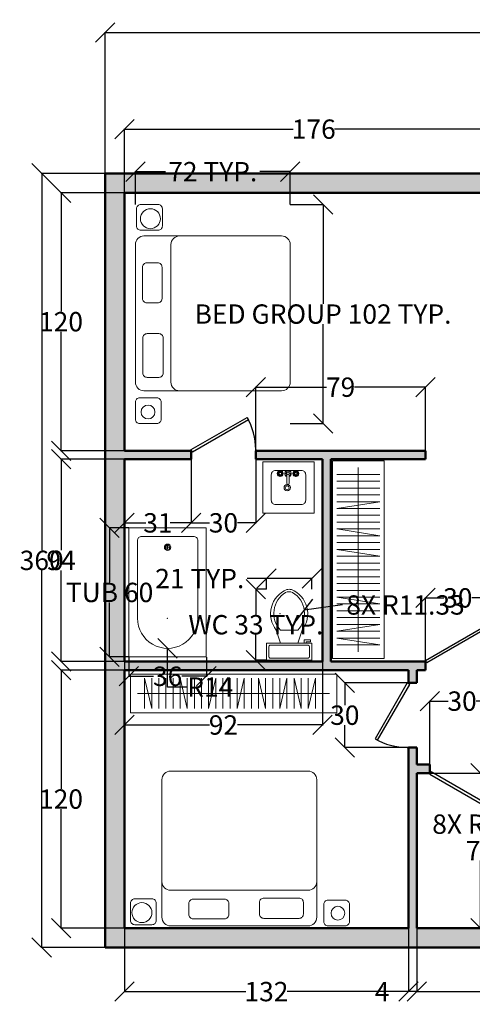
# Model space of a CAD drawing. Units: inches. Extents: x -9 to 615, y -420 to 89.
# Tile 1 of 6: x -9 to 201, y -368 to 89. Entities that reach past the tile are written whole.
import ezdxf

# ---------------------------------------------------------------- set-up
doc = ezdxf.new("R2010")
doc.units = ezdxf.units.IN
doc.header["$MEASUREMENT"] = 0
for name, color, linetype, lineweight in [('A-ANNO-DIMS', 2, 'Continuous', 18), ('A-DOOR', 4, 'Continuous', 25), ('A-FLOR-CASE', 32, 'Continuous', 18), ('A-FLOR-FIXT', 9, 'Continuous', 18), ('A-FURN', 8, 'Continuous', 18), ('A-WALL', 7, 'Continuous', 50)]:
    doc.layers.add(name, color=color, linetype=linetype, lineweight=lineweight)
doc.layers.add('A-WALL-PATT', color=251, linetype='Continuous', lineweight=13, true_color=0x636466)
doc.styles.get("Standard").update_dxf_attribs({"font": 'arial.ttf'})
doc.dimstyles.get("Standard").update_dxf_attribs({"dimtxt": 9, "dimasz": 9, "dimexe": 0.18, "dimexo": 0.0625, "dimgap": 0.09, "dimtad": 0, "dimtih": 1, "dimtoh": 1, "dimdec": 0, "dimzin": 0, "dimdsep": 46, "dimlunit": 4, "dimtxsty": 'Standard', "dimblk": 'OBLIQUE', "dimblk2": 'OBLIQUE', "dimcen": 0.09, "dimadec": 0, "dimazin": 0, "dimtfac": 1, "dimtdec": 0, "dimtofl": 0, "dimtmove": 0, "dimatfit": 3, "dimldrblk": 'OBLIQUE', "dimfxl": 1, "dimtolj": 1, "dimtzin": 0, "dimarcsym": 0})

# ---------------------------------------------------------------- blocks, each defined once
blk = doc.blocks.new('6 BED')
for p, q in [((-33.45, 25.64), (30.55, 25.64)), ((-37.45, 21.64), (-37.45, -23.43)), ((34.55, 21.64), (34.55, -19.64))]:
    blk.add_line(p, q)
for points in [[(-42.69, 42.2), (-50.69, 42.2, 0.414214), (-52.69, 40.2), (-52.69, 32.2, 0.414214), (-50.69, 30.2), (-42.69, 30.2, 0.414214), (-40.69, 32.2), (-40.69, 40.2, 0.414214)], [(-33.45, 42.2), (30.55, 42.2, -0.414214), (34.55, 38.2), (34.55, -25.8, -0.414214), (30.55, -29.8), (-33.45, -29.8, -0.414214), (-37.45, -25.8), (-37.45, 38.2, -0.414214)], [(39.19, 41.65), (47.19, 41.65, -0.414214), (49.19, 39.65), (49.19, 31.65, -0.414214), (47.19, 29.65), (39.19, 29.65, -0.414214), (37.19, 31.65), (37.19, 39.65, -0.414214)], [(-29.22, 38.71), (-12.85, 38.71, -0.414214), (-10.85, 36.71), (-10.85, 31.26, -0.414214), (-12.85, 29.26), (-29.22, 29.26, -0.414214), (-31.22, 31.26), (-31.22, 36.71, -0.414214)], [(5.45, 38.89), (20.03, 38.89, -0.414214), (22.03, 36.89), (22.03, 31.79, -0.414214), (20.03, 29.79), (5.45, 29.79, -0.414214), (3.45, 31.79), (3.45, 36.89, -0.414214)]]:
    blk.add_lwpolyline(points, format="xyb", close=True)
for centre, start, end in [((-33.45, 21.64), 90, 180), ((30.55, 21.64), 0, 90)]:
    blk.add_arc(centre, 4, start, end)
blk = doc.blocks.new('Bath Tub - 26 x 60 in.')
for p, q in [((8, -18), (10, -18)), ((9, -17), (9, -19))]:
    blk.add_line(p, q)
blk.add_lwpolyline([(0, -36), (0, 0), (60, 0), (60, -36)], close=True)
for points in [[(6, -4), (42, -4)], [(4, -30), (4, -6)], [(42, -32), (6, -32)]]:
    blk.add_lwpolyline(points)
for radius in [1.5, 1]:
    blk.add_circle((9, -18), radius)
for centre, radius, start, end in [((5.75, -5.75), 1.77, 81.8699, 188.1301), ((42, -18), 14, 270, 90), ((5.75, -30.25), 1.77, 171.8699, 278.1301)]:
    blk.add_arc(centre, radius, start, end)
blk = doc.blocks.new('Toilet - top')
for p, q in [((9.5, -6), (9.5, -2)), ((-10, -8.5), (-8, -8.5)), ((-10, -9.5), (-10, -8.5)), ((-8, -8.5), (-8, -8)), ((-7, -8), (-7, -9.5)), ((-4, -8), (-6, -14)), ((4, -8), (6, -14)), ((-7, -9.5), (-10, -9.5)), ((4, -14), (-4, -14))]:
    blk.add_line(p, q)
blk.add_lwpolyline([(10.5, -8), (10.5, 0), (-10.5, 0), (-10.5, -8)], close=True)
for points in [[(-9.5, -2), (-9.5, -6)], [(8.5, -1), (-8.5, -1)], [(-8.5, -7), (8.5, -7)]]:
    blk.add_lwpolyline(points)
for centre, radius, start, end in [((-8.62, -1.88), 0.884, 81.8699, 188.1301), ((8.62, -1.88), 0.884, 351.8699, 98.1301), ((-8.62, -6.12), 0.884, 171.8699, 278.1301), ((8.62, -6.12), 0.884, 261.8699, 8.1301), ((3.52, -21.58), 12.17, 141.4691, 247.9714), ((4.2, -21.82), 11.33, 136.3677, 238.9468), ((-3.52, -21.58), 12.17, 292.0284, 38.5307), ((-4.2, -21.82), 11.33, 301.053, 43.6321), ((0, -27.88), 4, 245.7318, 294.2682), ((0, -29), 4, 254.8605, 285.1395)]:
    blk.add_arc(centre, radius, start, end)
blk = doc.blocks.new('*U12')
for p, q in [((0, 0), (0, -6)), ((40, 0), (40, -6))]:
    blk.add_line(p, q)
blk.add_lwpolyline([(0, 0), (34.64, 20), (35.52, 18.48), (0.87, -1.52)], close=True)
blk.add_arc((0, 0), 40, 0, 30)
blk = doc.blocks.new('*U13')
for p, q in [((0, 0), (0, 6)), ((40, 0), (40, 6))]:
    blk.add_line(p, q)
blk.add_lwpolyline([(0, 0), (34.64, -20), (35.52, -18.48), (0.87, 1.52)], close=True)
blk.add_arc((0, 0), 40, 330, 0)
blk = doc.blocks.new('Faucet - Bathroom top')
for p, q in [((-4.107, 0.125), (-4.375, 0.125)), ((-3.75, 0.4788), (-3.75, 0.75)), ((-3.5, 0.482), (-3.5, 0.75)), ((-3.1461, 0.125), (-2.875, 0.125)), ((3.143, 0.125), (2.875, 0.125)), ((3.5, 0.4788), (3.5, 0.75)), ((3.75, 0.482), (3.75, 0.75)), ((4.1039, 0.125), (4.375, 0.125)), ((-4.1039, -0.125), (-4.375, -0.125)), ((-3.75, -0.4821), (-3.75, -0.75)), ((-3.5, -0.4789), (-3.5, -0.75)), ((-3.143, -0.125), (-2.875, -0.125)), ((-0.5, -0.8639), (-0.5, -4.5)), ((0.5, -4.5), (0.5, -0.8631)), ((3.1461, -0.125), (2.875, -0.125)), ((3.5, -0.4821), (3.5, -0.75)), ((3.75, -0.4789), (3.75, -0.75)), ((4.107, -0.125), (4.375, -0.125))]:
    blk.add_line(p, q)
for centre, radius in [((-3.625, 0), 1.375), ((-4.625, 0), 0.2795), ((-3.625, 0), 0.5), ((-3.625, 1), 0.2795), ((-2.625, 0), 0.2795), ((0, 0), 0.5), ((3.625, 0), 1.375), ((2.625, 0), 0.2795), ((3.625, 0), 0.5), ((3.625, 1), 0.2795), ((4.625, 0), 0.2795), ((-3.625, -1), 0.2795), ((3.625, -1), 0.2795)]:
    blk.add_circle(centre, radius)
for centre, radius, start, end in [((-3.625, 0), 1, 105.2407, 164.2093), ((-3.625, 0), 1, 16.44125, 74.07887), ((0, 0), 1.5, 289.6514, 250.3603), ((0, 0), 1, 300.3431, 239.7554), ((3.625, 0), 1, 106.12, 164.0884), ((3.625, 0), 1, 16.23422, 73.90469), ((-3.625, 0), 1, 196.2342, 253.9047), ((-3.625, 0), 1, 286.12, 344.0884), ((0, -4.5), 0.5, 180, 0), ((3.625, 0), 1, 196.4413, 254.0789), ((3.625, 0), 1, 285.2407, 344.2093)]:
    blk.add_arc(centre, radius, start, end)
blk = doc.blocks.new('LAVATORY-24IN')
blk.add_lwpolyline([(0, 23.91), (0, 0), (24, 0), (24, 23.91)], close=True)
blk.add_lwpolyline([(4, 17.91), (4, 6, 0.414214), (6, 4), (18, 4, 0.414214), (20, 6), (20, 17.91, 0.414214), (18, 19.91), (6, 19.91, 0.414214)], format="xyb", close=True)
for centre, radius in [((11.41, 11.89), 1.47), ((11.39, 11.82), 0.91)]:
    blk.add_circle(centre, radius)
blk.add_blockref('Faucet - Bathroom top', (11.81, 18.42))
blk = doc.blocks.new('_Oblique')
at = {"color": 0, "linetype": 'ByBlock', "lineweight": -2}
blk.add_line((-0.5, -0.5), (0.5, 0.5), dxfattribs=at)
blk = doc.blocks.new('*D18')
at = {"layer": 'A-ANNO-DIMS', "color": 0, "lineweight": -2, "transparency": 16777216}
for p, q in [((116.54, 3.51), (131.94, 3.51)), ((131.76, 3.51), (131.76, -42.68)), ((131.76, -98.36), (131.76, -52.17)), ((116.54, -98.36), (131.94, -98.36))]:
    blk.add_line(p, q, dxfattribs=at)
at = {"layer": 'Defpoints', "color": 0, "transparency": 16777216}
for p in [(116.47, 3.51), (131.76, 3.51), (116.47, -98.36)]:
    blk.add_point(p, dxfattribs=at)
at = {"layer": 'A-ANNO-DIMS', "color": 0, "lineweight": -2, "transparency": 16777216, "xscale": 9, "yscale": 9, "zscale": 9}
for p, rotation in [((131.76, 3.51), 90), ((131.76, -98.36), 270)]:
    blk.add_blockref('_Oblique', p, dxfattribs=dict(at, rotation=rotation))
at = {"layer": 'A-ANNO-DIMS', "color": 0, "transparency": 16777216, "insert": (131.76, -47.43), "char_height": 9, "attachment_point": 5}
blk.add_mtext('\\A1;BED GROUP 102 TYP.', dxfattribs=at)
blk = doc.blocks.new('*D19')
at = {"layer": 'A-ANNO-DIMS', "color": 0, "lineweight": -2, "transparency": 16777216}
for p, q in [((44.47, 3.58), (44.47, 18.98)), ((44.47, 18.8), (58.52, 18.8)), ((116.47, 18.8), (102.43, 18.8)), ((116.47, 3.58), (116.47, 18.98))]:
    blk.add_line(p, q, dxfattribs=at)
at = {"layer": 'Defpoints', "color": 0, "transparency": 16777216}
for p in [(44.47, 18.8), (44.47, 3.51), (116.47, 3.51)]:
    blk.add_point(p, dxfattribs=at)
at = {"layer": 'A-ANNO-DIMS', "color": 0, "lineweight": -2, "transparency": 16777216, "xscale": 9, "yscale": 9, "zscale": 9, "rotation": 180}
blk.add_blockref('_Oblique', (44.47, 18.8), dxfattribs=at)
at = {"layer": 'A-ANNO-DIMS', "color": 0, "lineweight": -2, "transparency": 16777216, "xscale": 9, "yscale": 9, "zscale": 9}
blk.add_blockref('_Oblique', (116.47, 18.8), dxfattribs=at)
at = {"layer": 'A-ANNO-DIMS', "color": 0, "transparency": 16777216, "insert": (80.47, 18.8), "char_height": 9, "attachment_point": 5}
blk.add_mtext('\\A1;72 TYP.', dxfattribs=at)
blk = doc.blocks.new('*D20')
at = {"layer": 'A-ANNO-DIMS', "color": 0, "lineweight": -2, "transparency": 16777216}
for p, q in [((105.43, -175.39), (100.35, -175.39)), ((100.53, -175.39), (100.53, -187.17)), ((100.53, -208.43), (100.53, -196.66)), ((105.43, -208.43), (100.35, -208.43))]:
    blk.add_line(p, q, dxfattribs=at)
at = {"layer": 'Defpoints', "color": 0, "transparency": 16777216}
for p in [(105.49, -175.39), (100.53, -208.43), (105.49, -208.43)]:
    blk.add_point(p, dxfattribs=at)
at = {"layer": 'A-ANNO-DIMS', "color": 0, "lineweight": -2, "transparency": 16777216, "xscale": 9, "yscale": 9, "zscale": 9}
for p, rotation in [((100.53, -175.39), 90), ((100.53, -208.43), 270)]:
    blk.add_blockref('_Oblique', p, dxfattribs=dict(at, rotation=rotation))
at = {"layer": 'A-ANNO-DIMS', "color": 0, "transparency": 16777216, "insert": (100.53, -191.91), "char_height": 9, "attachment_point": 5}
blk.add_mtext('\\A1;WC 33 TYP.', dxfattribs=at)
blk = doc.blocks.new('*D21')
at = {"layer": 'A-ANNO-DIMS', "color": 0, "lineweight": -2, "transparency": 16777216}
for p, q in [((105.49, -170.43), (96.49, -170.43)), ((105.49, -175.33), (105.49, -170.25)), ((126.49, -170.43), (105.49, -170.43)), ((126.49, -175.33), (126.49, -170.25))]:
    blk.add_line(p, q, dxfattribs=at)
at = {"layer": 'Defpoints', "color": 0, "transparency": 16777216}
for p in [(105.49, -170.43), (105.49, -175.39), (126.49, -175.39)]:
    blk.add_point(p, dxfattribs=at)
at = {"layer": 'A-ANNO-DIMS', "color": 0, "lineweight": -2, "transparency": 16777216, "xscale": 9, "yscale": 9, "zscale": 9, "rotation": 180}
blk.add_blockref('_Oblique', (105.49, -170.43), dxfattribs=at)
at = {"layer": 'A-ANNO-DIMS', "color": 0, "lineweight": -2, "transparency": 16777216, "xscale": 9, "yscale": 9, "zscale": 9}
blk.add_blockref('_Oblique', (126.49, -170.43), dxfattribs=at)
at = {"layer": 'A-ANNO-DIMS', "color": 0, "transparency": 16777216, "insert": (74.42, -170.43), "char_height": 9, "attachment_point": 5}
blk.add_mtext('\\A1;21 TYP.', dxfattribs=at)
blk = doc.blocks.new('*D36')
at = {"layer": 'A-ANNO-DIMS', "color": 0, "lineweight": -2, "transparency": 16777216}
for p, q in [((41.41, -146.89), (32.3, -146.89)), ((32.48, -146.89), (32.48, -172.2)), ((32.48, -206.89), (32.48, -181.57)), ((41.41, -206.89), (32.3, -206.89))]:
    blk.add_line(p, q, dxfattribs=at)
at = {"layer": 'Defpoints', "color": 0, "transparency": 16777216}
for p in [(41.48, -146.89), (32.48, -206.89), (41.48, -206.89)]:
    blk.add_point(p, dxfattribs=at)
at = {"layer": 'A-ANNO-DIMS', "color": 0, "lineweight": -2, "transparency": 16777216, "xscale": 9, "yscale": 9, "zscale": 9}
for p, rotation in [((32.48, -146.89), 90), ((32.48, -206.89), 270)]:
    blk.add_blockref('_Oblique', p, dxfattribs=dict(at, rotation=rotation))
at = {"layer": 'A-ANNO-DIMS', "color": 0, "transparency": 16777216, "insert": (32.48, -176.89), "char_height": 9, "attachment_point": 5}
blk.add_mtext('\\A1;TUB 60', dxfattribs=at)
blk = doc.blocks.new('*D37')
at = {"layer": 'A-ANNO-DIMS', "color": 0, "lineweight": -2, "transparency": 16777216}
for p, q in [((41.48, -206.95), (41.48, -216.07)), ((77.48, -206.95), (77.48, -216.07)), ((41.48, -215.89), (52.95, -215.89)), ((77.48, -215.89), (66.01, -215.89))]:
    blk.add_line(p, q, dxfattribs=at)
at = {"layer": 'Defpoints', "color": 0, "transparency": 16777216}
for p in [(41.48, -206.89), (77.48, -206.89), (77.48, -215.89)]:
    blk.add_point(p, dxfattribs=at)
at = {"layer": 'A-ANNO-DIMS', "color": 0, "lineweight": -2, "transparency": 16777216, "xscale": 9, "yscale": 9, "zscale": 9, "rotation": 180}
blk.add_blockref('_Oblique', (41.48, -215.89), dxfattribs=at)
at = {"layer": 'A-ANNO-DIMS', "color": 0, "lineweight": -2, "transparency": 16777216, "xscale": 9, "yscale": 9, "zscale": 9}
blk.add_blockref('_Oblique', (77.48, -215.89), dxfattribs=at)
at = {"layer": 'A-ANNO-DIMS', "color": 0, "transparency": 16777216, "insert": (59.48, -215.89), "char_height": 9, "attachment_point": 5}
blk.add_mtext('\\A1;36', dxfattribs=at)
blk = doc.blocks.new('*D40')
at = {"layer": 'A-ANNO-DIMS', "color": 0, "lineweight": -2, "transparency": 16777216}
for p, q in [((30.44, 18.08), (30.44, 83.75)), ((30.44, 83.57), (290.42, 83.57)), ((570.44, 83.57), (310.45, 83.57)), ((570.44, 18.08), (570.44, 83.75))]:
    blk.add_line(p, q, dxfattribs=at)
at = {"layer": 'Defpoints', "color": 0, "transparency": 16777216}
for p in [(570.44, 83.57), (30.44, 18.02), (570.44, 18.02)]:
    blk.add_point(p, dxfattribs=at)
at = {"layer": 'A-ANNO-DIMS', "color": 0, "lineweight": -2, "transparency": 16777216, "xscale": 9, "yscale": 9, "zscale": 9, "rotation": 180}
blk.add_blockref('_Oblique', (30.44, 83.57), dxfattribs=at)
at = {"layer": 'A-ANNO-DIMS', "color": 0, "lineweight": -2, "transparency": 16777216, "xscale": 9, "yscale": 9, "zscale": 9}
blk.add_blockref('_Oblique', (570.44, 83.57), dxfattribs=at)
at = {"layer": 'A-ANNO-DIMS', "color": 0, "transparency": 16777216, "insert": (300.44, 83.57), "char_height": 9, "attachment_point": 5}
blk.add_mtext('\\A1;540', dxfattribs=at)
blk = doc.blocks.new('*D41')
at = {"layer": 'A-ANNO-DIMS', "color": 0, "lineweight": -2, "transparency": 16777216}
for p, q in [((30.38, 18.02), (0.71, 18.02)), ((0.89, 18.02), (0.89, -157.29)), ((0.89, -341.98), (0.89, -166.67)), ((30.38, -341.98), (0.71, -341.98))]:
    blk.add_line(p, q, dxfattribs=at)
at = {"layer": 'Defpoints', "color": 0, "transparency": 16777216}
for p in [(0.89, 18.02), (30.44, 18.02), (30.44, -341.98)]:
    blk.add_point(p, dxfattribs=at)
at = {"layer": 'A-ANNO-DIMS', "color": 0, "lineweight": -2, "transparency": 16777216, "xscale": 9, "yscale": 9, "zscale": 9}
for p, rotation in [((0.89, 18.02), 90), ((0.89, -341.98), 270)]:
    blk.add_blockref('_Oblique', p, dxfattribs=dict(at, rotation=rotation))
at = {"layer": 'A-ANNO-DIMS', "color": 0, "transparency": 16777216, "insert": (0.89, -161.98), "char_height": 9, "attachment_point": 5}
blk.add_mtext('\\A1;360', dxfattribs=at)
blk = doc.blocks.new('*D43')
at = {"layer": 'A-ANNO-DIMS', "color": 0, "lineweight": -2, "transparency": 16777216}
for p, q in [((39.44, 9.08), (39.44, 38.75)), ((39.44, 38.57), (117.83, 38.57)), ((215.44, 38.57), (137.04, 38.57)), ((215.44, 9.08), (215.44, 38.75))]:
    blk.add_line(p, q, dxfattribs=at)
at = {"layer": 'Defpoints', "color": 0, "transparency": 16777216}
for p in [(215.44, 38.57), (39.44, 9.02), (215.44, 9.02)]:
    blk.add_point(p, dxfattribs=at)
at = {"layer": 'A-ANNO-DIMS', "color": 0, "lineweight": -2, "transparency": 16777216, "xscale": 9, "yscale": 9, "zscale": 9, "rotation": 180}
blk.add_blockref('_Oblique', (39.44, 38.57), dxfattribs=at)
at = {"layer": 'A-ANNO-DIMS', "color": 0, "lineweight": -2, "transparency": 16777216, "xscale": 9, "yscale": 9, "zscale": 9}
blk.add_blockref('_Oblique', (215.44, 38.57), dxfattribs=at)
at = {"layer": 'A-ANNO-DIMS', "color": 0, "transparency": 16777216, "insert": (127.44, 38.57), "char_height": 9, "attachment_point": 5}
blk.add_mtext('\\A1;176', dxfattribs=at)
blk = doc.blocks.new('*D49')
at = {"layer": 'A-ANNO-DIMS', "color": 0, "lineweight": -2, "transparency": 16777216}
for p, q in [((39.44, -333.04), (39.44, -362.71)), ((171.44, -333.04), (171.44, -362.71)), ((39.44, -362.53), (95.88, -362.53)), ((171.44, -362.53), (115, -362.53))]:
    blk.add_line(p, q, dxfattribs=at)
at = {"layer": 'Defpoints', "color": 0, "transparency": 16777216}
for p in [(39.44, -332.98), (171.44, -332.98), (39.44, -362.53)]:
    blk.add_point(p, dxfattribs=at)
at = {"layer": 'A-ANNO-DIMS', "color": 0, "lineweight": -2, "transparency": 16777216, "xscale": 9, "yscale": 9, "zscale": 9}
for p, rotation in [((39.44, -362.53), 179.9999999999999), ((171.44, -362.53), 359.9999999999999)]:
    blk.add_blockref('_Oblique', p, dxfattribs=dict(at, rotation=rotation))
at = {"layer": 'A-ANNO-DIMS', "color": 0, "transparency": 16777216, "insert": (105.44, -362.53), "char_height": 9, "attachment_point": 5}
blk.add_mtext('\\A1;132', dxfattribs=at)
blk = doc.blocks.new('*D50')
at = {"layer": 'A-ANNO-DIMS', "color": 0, "lineweight": -2, "transparency": 16777216}
for p, q in [((175.44, -333.04), (175.44, -362.71)), ((279.44, -333.04), (279.44, -362.71)), ((175.44, -362.53), (217.85, -362.53)), ((279.44, -362.53), (237.03, -362.53))]:
    blk.add_line(p, q, dxfattribs=at)
at = {"layer": 'Defpoints', "color": 0, "transparency": 16777216}
for p in [(175.44, -332.98), (279.44, -332.98), (175.44, -362.53)]:
    blk.add_point(p, dxfattribs=at)
at = {"layer": 'A-ANNO-DIMS', "color": 0, "lineweight": -2, "transparency": 16777216, "xscale": 9, "yscale": 9, "zscale": 9, "rotation": 180}
blk.add_blockref('_Oblique', (175.44, -362.53), dxfattribs=at)
at = {"layer": 'A-ANNO-DIMS', "color": 0, "lineweight": -2, "transparency": 16777216, "xscale": 9, "yscale": 9, "zscale": 9}
blk.add_blockref('_Oblique', (279.44, -362.53), dxfattribs=at)
at = {"layer": 'A-ANNO-DIMS', "color": 0, "transparency": 16777216, "insert": (227.44, -362.53), "char_height": 9, "attachment_point": 5}
blk.add_mtext('\\A1;104', dxfattribs=at)
blk = doc.blocks.new('*D55')
at = {"layer": 'A-ANNO-DIMS', "color": 0, "lineweight": -2, "transparency": 16777216}
for p, q in [((39.38, 9.02), (9.71, 9.02)), ((9.89, 9.02), (9.89, -46.3)), ((9.89, -110.98), (9.89, -55.67)), ((39.38, -110.98), (9.71, -110.98))]:
    blk.add_line(p, q, dxfattribs=at)
at = {"layer": 'Defpoints', "color": 0, "transparency": 16777216}
for p in [(9.89, 9.02), (39.44, 9.02), (39.44, -110.98)]:
    blk.add_point(p, dxfattribs=at)
at = {"layer": 'A-ANNO-DIMS', "color": 0, "lineweight": -2, "transparency": 16777216, "xscale": 9, "yscale": 9, "zscale": 9}
for p, rotation in [((9.89, 9.02), 90), ((9.89, -110.98), 270)]:
    blk.add_blockref('_Oblique', p, dxfattribs=dict(at, rotation=rotation))
at = {"layer": 'A-ANNO-DIMS', "color": 0, "transparency": 16777216, "insert": (9.89, -50.98), "char_height": 9, "attachment_point": 5}
blk.add_mtext('\\A1;120', dxfattribs=at)
blk = doc.blocks.new('*D56')
at = {"layer": 'A-ANNO-DIMS', "color": 0, "lineweight": -2, "transparency": 16777216}
for p, q in [((39.38, -114.98), (9.71, -114.98)), ((9.89, -114.98), (9.89, -157.3)), ((9.89, -208.98), (9.89, -166.67)), ((39.38, -208.98), (9.71, -208.98))]:
    blk.add_line(p, q, dxfattribs=at)
at = {"layer": 'Defpoints', "color": 0, "transparency": 16777216}
for p in [(9.89, -114.98), (39.44, -114.98), (39.44, -208.98)]:
    blk.add_point(p, dxfattribs=at)
at = {"layer": 'A-ANNO-DIMS', "color": 0, "lineweight": -2, "transparency": 16777216, "xscale": 9, "yscale": 9, "zscale": 9}
for p, rotation in [((9.89, -114.98), 90), ((9.89, -208.98), 270)]:
    blk.add_blockref('_Oblique', p, dxfattribs=dict(at, rotation=rotation))
at = {"layer": 'A-ANNO-DIMS', "color": 0, "transparency": 16777216, "insert": (9.89, -161.98), "char_height": 9, "attachment_point": 5}
blk.add_mtext('\\A1;94', dxfattribs=at)
blk = doc.blocks.new('*D57')
at = {"layer": 'A-ANNO-DIMS', "color": 0, "lineweight": -2, "transparency": 16777216}
for p, q in [((39.38, -212.98), (9.71, -212.98)), ((9.89, -212.98), (9.89, -268.3)), ((9.89, -332.98), (9.89, -277.67)), ((39.38, -332.98), (9.71, -332.98))]:
    blk.add_line(p, q, dxfattribs=at)
at = {"layer": 'Defpoints', "color": 0, "transparency": 16777216}
for p in [(9.89, -212.98), (39.44, -212.98), (39.44, -332.98)]:
    blk.add_point(p, dxfattribs=at)
at = {"layer": 'A-ANNO-DIMS', "color": 0, "lineweight": -2, "transparency": 16777216, "xscale": 9, "yscale": 9, "zscale": 9}
for p, rotation in [((9.89, -212.98), 90), ((9.89, -332.98), 270)]:
    blk.add_blockref('_Oblique', p, dxfattribs=dict(at, rotation=rotation))
at = {"layer": 'A-ANNO-DIMS', "color": 0, "transparency": 16777216, "insert": (9.89, -272.98), "char_height": 9, "attachment_point": 5}
blk.add_mtext('\\A1;120', dxfattribs=at)
blk = doc.blocks.new('*D60')
at = {"layer": 'A-ANNO-DIMS', "color": 0, "lineweight": -2, "transparency": 16777216}
for p, q in [((39.44, -209.04), (39.44, -238.71)), ((131.44, -209.04), (131.44, -238.71)), ((39.44, -238.53), (78.95, -238.53)), ((131.44, -238.53), (91.93, -238.53))]:
    blk.add_line(p, q, dxfattribs=at)
at = {"layer": 'Defpoints', "color": 0, "transparency": 16777216}
for p in [(39.44, -208.98), (131.44, -208.98), (39.44, -238.53)]:
    blk.add_point(p, dxfattribs=at)
at = {"layer": 'A-ANNO-DIMS', "color": 0, "lineweight": -2, "transparency": 16777216, "xscale": 9, "yscale": 9, "zscale": 9, "rotation": 180}
blk.add_blockref('_Oblique', (39.44, -238.53), dxfattribs=at)
at = {"layer": 'A-ANNO-DIMS', "color": 0, "lineweight": -2, "transparency": 16777216, "xscale": 9, "yscale": 9, "zscale": 9}
blk.add_blockref('_Oblique', (131.44, -238.53), dxfattribs=at)
at = {"layer": 'A-ANNO-DIMS', "color": 0, "transparency": 16777216, "insert": (85.44, -238.53), "char_height": 9, "attachment_point": 5}
blk.add_mtext('\\A1;92', dxfattribs=at)
blk = doc.blocks.new('*D62')
at = {"layer": 'A-ANNO-DIMS', "color": 0, "lineweight": -2, "transparency": 16777216}
for p, q in [((175.5, -260.98), (205.17, -260.98)), ((204.99, -260.98), (204.99, -292.37)), ((204.99, -332.98), (204.99, -301.59)), ((175.5, -332.98), (205.17, -332.98))]:
    blk.add_line(p, q, dxfattribs=at)
at = {"layer": 'Defpoints', "color": 0, "transparency": 16777216}
for p in [(175.44, -260.98), (175.44, -332.98), (204.99, -332.98)]:
    blk.add_point(p, dxfattribs=at)
at = {"layer": 'A-ANNO-DIMS', "color": 0, "lineweight": -2, "transparency": 16777216, "xscale": 9, "yscale": 9, "zscale": 9}
for p, rotation in [((204.99, -260.98), 90), ((204.99, -332.98), 270)]:
    blk.add_blockref('_Oblique', p, dxfattribs=dict(at, rotation=rotation))
at = {"layer": 'A-ANNO-DIMS', "color": 0, "transparency": 16777216, "insert": (204.99, -296.98), "char_height": 9, "attachment_point": 5}
blk.add_mtext('\\A1;72', dxfattribs=at)
blk = doc.blocks.new('*D66')
at = {"layer": 'A-ANNO-DIMS', "color": 0, "lineweight": -2, "transparency": 16777216}
for p, q in [((171.44, -333.04), (171.44, -362.71)), ((175.44, -333.04), (175.44, -362.71)), ((171.44, -362.53), (162.44, -362.53)), ((175.44, -362.53), (171.44, -362.53))]:
    blk.add_line(p, q, dxfattribs=at)
at = {"layer": 'Defpoints', "color": 0, "transparency": 16777216}
for p in [(171.44, -332.98), (175.44, -332.98), (171.44, -362.53)]:
    blk.add_point(p, dxfattribs=at)
at = {"layer": 'A-ANNO-DIMS', "color": 0, "lineweight": -2, "transparency": 16777216, "xscale": 9, "yscale": 9, "zscale": 9}
for p, rotation in [((171.44, -362.53), 180.0000000000016), ((175.44, -362.53), 1.5987e-12)]:
    blk.add_blockref('_Oblique', p, dxfattribs=dict(at, rotation=rotation))
at = {"layer": 'A-ANNO-DIMS', "color": 0, "transparency": 16777216, "insert": (159.24, -362.53), "char_height": 9, "attachment_point": 5}
blk.add_mtext('\\A1;4', dxfattribs=at)
blk = doc.blocks.new('*D74')
at = {"layer": 'A-ANNO-DIMS', "color": 0, "lineweight": -2, "transparency": 16777216}
for p, q in [((39.44, -115.04), (39.44, -144.71)), ((70.44, -115.04), (70.44, -144.71)), ((39.44, -144.53), (49.27, -144.53)), ((70.44, -144.53), (60.6, -144.53))]:
    blk.add_line(p, q, dxfattribs=at)
at = {"layer": 'Defpoints', "color": 0, "transparency": 16777216}
for p in [(39.44, -114.98), (70.44, -114.98), (39.44, -144.53)]:
    blk.add_point(p, dxfattribs=at)
at = {"layer": 'A-ANNO-DIMS', "color": 0, "lineweight": -2, "transparency": 16777216, "xscale": 9, "yscale": 9, "zscale": 9, "rotation": 180}
blk.add_blockref('_Oblique', (39.44, -144.53), dxfattribs=at)
at = {"layer": 'A-ANNO-DIMS', "color": 0, "lineweight": -2, "transparency": 16777216, "xscale": 9, "yscale": 9, "zscale": 9}
blk.add_blockref('_Oblique', (70.44, -144.53), dxfattribs=at)
at = {"layer": 'A-ANNO-DIMS', "color": 0, "transparency": 16777216, "insert": (54.94, -144.53), "char_height": 9, "attachment_point": 5}
blk.add_mtext('\\A1;31', dxfattribs=at)
blk = doc.blocks.new('*D75')
at = {"layer": 'A-ANNO-DIMS', "color": 0, "lineweight": -2, "transparency": 16777216}
for p, q in [((70.44, -115.04), (70.44, -144.71)), ((100.44, -115.04), (100.44, -144.71)), ((70.44, -144.53), (78.92, -144.53)), ((100.44, -144.53), (91.96, -144.53))]:
    blk.add_line(p, q, dxfattribs=at)
at = {"layer": 'Defpoints', "color": 0, "transparency": 16777216}
for p in [(70.44, -114.98), (100.44, -114.98), (70.44, -144.53)]:
    blk.add_point(p, dxfattribs=at)
at = {"layer": 'A-ANNO-DIMS', "color": 0, "lineweight": -2, "transparency": 16777216, "xscale": 9, "yscale": 9, "zscale": 9, "rotation": 180.0000000000002}
blk.add_blockref('_Oblique', (70.44, -144.53), dxfattribs=at)
at = {"layer": 'A-ANNO-DIMS', "color": 0, "lineweight": -2, "transparency": 16777216, "xscale": 9, "yscale": 9, "zscale": 9}
blk.add_blockref('_Oblique', (100.44, -144.53), dxfattribs=at)
at = {"layer": 'A-ANNO-DIMS', "color": 0, "transparency": 16777216, "insert": (85.44, -144.53), "char_height": 9, "attachment_point": 5}
blk.add_mtext('\\A1;30', dxfattribs=at)
blk = doc.blocks.new('*D76')
at = {"layer": 'A-ANNO-DIMS', "color": 0, "lineweight": -2, "transparency": 16777216}
for p, q in [((100.44, -110.92), (100.44, -81.25)), ((100.44, -81.43), (133.43, -81.43)), ((179.44, -81.43), (146.45, -81.43)), ((179.44, -110.92), (179.44, -81.25))]:
    blk.add_line(p, q, dxfattribs=at)
at = {"layer": 'Defpoints', "color": 0, "transparency": 16777216}
for p in [(179.44, -81.43), (100.44, -110.98), (179.44, -110.98)]:
    blk.add_point(p, dxfattribs=at)
at = {"layer": 'A-ANNO-DIMS', "color": 0, "lineweight": -2, "transparency": 16777216, "xscale": 9, "yscale": 9, "zscale": 9, "rotation": 180}
blk.add_blockref('_Oblique', (100.44, -81.43), dxfattribs=at)
at = {"layer": 'A-ANNO-DIMS', "color": 0, "lineweight": -2, "transparency": 16777216, "xscale": 9, "yscale": 9, "zscale": 9}
blk.add_blockref('_Oblique', (179.44, -81.43), dxfattribs=at)
at = {"layer": 'A-ANNO-DIMS', "color": 0, "transparency": 16777216, "insert": (139.94, -81.43), "char_height": 9, "attachment_point": 5}
blk.add_mtext('\\A1;79', dxfattribs=at)
blk = doc.blocks.new('*D77')
at = {"layer": 'A-ANNO-DIMS', "color": 0, "lineweight": -2, "transparency": 16777216}
for p, q in [((179.44, -208.92), (179.44, -179.25)), ((179.44, -179.43), (187.92, -179.43)), ((209.44, -179.43), (200.96, -179.43)), ((209.44, -208.92), (209.44, -179.25))]:
    blk.add_line(p, q, dxfattribs=at)
at = {"layer": 'Defpoints', "color": 0, "transparency": 16777216}
for p in [(209.44, -179.43), (179.44, -208.98), (209.44, -208.98)]:
    blk.add_point(p, dxfattribs=at)
at = {"layer": 'A-ANNO-DIMS', "color": 0, "lineweight": -2, "transparency": 16777216, "xscale": 9, "yscale": 9, "zscale": 9, "rotation": 180}
blk.add_blockref('_Oblique', (179.44, -179.43), dxfattribs=at)
at = {"layer": 'A-ANNO-DIMS', "color": 0, "lineweight": -2, "transparency": 16777216, "xscale": 9, "yscale": 9, "zscale": 9}
blk.add_blockref('_Oblique', (209.44, -179.43), dxfattribs=at)
at = {"layer": 'A-ANNO-DIMS', "color": 0, "transparency": 16777216, "insert": (194.44, -179.43), "char_height": 9, "attachment_point": 5}
blk.add_mtext('\\A1;30', dxfattribs=at)
blk = doc.blocks.new('*D79')
at = {"layer": 'A-ANNO-DIMS', "color": 0, "lineweight": -2, "transparency": 16777216}
for p, q in [((171.38, -218.98), (141.71, -218.98)), ((141.89, -218.98), (141.89, -229.29)), ((141.89, -248.98), (141.89, -238.67)), ((171.38, -248.98), (141.71, -248.98))]:
    blk.add_line(p, q, dxfattribs=at)
at = {"layer": 'Defpoints', "color": 0, "transparency": 16777216}
for p in [(141.89, -218.98), (171.44, -218.98), (171.44, -248.98)]:
    blk.add_point(p, dxfattribs=at)
at = {"layer": 'A-ANNO-DIMS', "color": 0, "lineweight": -2, "transparency": 16777216, "xscale": 9, "yscale": 9, "zscale": 9}
for p, rotation in [((141.89, -218.98), 90), ((141.89, -248.98), 270)]:
    blk.add_blockref('_Oblique', p, dxfattribs=dict(at, rotation=rotation))
at = {"layer": 'A-ANNO-DIMS', "color": 0, "transparency": 16777216, "insert": (141.89, -233.98), "char_height": 9, "attachment_point": 5}
blk.add_mtext('\\A1;30', dxfattribs=at)
blk = doc.blocks.new('*D80')
at = {"layer": 'A-ANNO-DIMS', "color": 0, "lineweight": -2, "transparency": 16777216}
for p, q in [((181.44, -256.92), (181.44, -227.25)), ((181.44, -227.43), (189.92, -227.43)), ((211.44, -227.43), (202.96, -227.43)), ((211.44, -256.92), (211.44, -227.25))]:
    blk.add_line(p, q, dxfattribs=at)
at = {"layer": 'Defpoints', "color": 0, "transparency": 16777216}
for p in [(211.44, -227.43), (181.44, -256.98), (211.44, -256.98)]:
    blk.add_point(p, dxfattribs=at)
at = {"layer": 'A-ANNO-DIMS', "color": 0, "lineweight": -2, "transparency": 16777216, "xscale": 9, "yscale": 9, "zscale": 9, "rotation": 180}
blk.add_blockref('_Oblique', (181.44, -227.43), dxfattribs=at)
at = {"layer": 'A-ANNO-DIMS', "color": 0, "lineweight": -2, "transparency": 16777216, "xscale": 9, "yscale": 9, "zscale": 9}
blk.add_blockref('_Oblique', (211.44, -227.43), dxfattribs=at)
at = {"layer": 'A-ANNO-DIMS', "color": 0, "transparency": 16777216, "insert": (196.44, -227.43), "char_height": 9, "attachment_point": 5}
blk.add_mtext('\\A1;30', dxfattribs=at)
blk = doc.blocks.new('*D91')
at = {"layer": 'A-ANNO-DIMS', "color": 0, "lineweight": -2, "transparency": 16777216}
for p, q in [((59.39, -188.89), (59.57, -188.89)), ((59.48, -188.98), (59.48, -188.8)), ((59.48, -220.89), (59.48, -202.89)), ((68.48, -220.89), (59.48, -220.89))]:
    blk.add_line(p, q, dxfattribs=at)
at = {"layer": 'Defpoints', "color": 0, "transparency": 16777216}
for p in [(59.48, -188.89), (59.48, -202.89)]:
    blk.add_point(p, dxfattribs=at)
at = {"layer": 'A-ANNO-DIMS', "color": 0, "lineweight": -2, "transparency": 16777216, "xscale": 9, "yscale": 9, "zscale": 9, "rotation": 90.00049519923718}
blk.add_blockref('_Oblique', (59.48, -202.89), dxfattribs=at)
at = {"layer": 'A-ANNO-DIMS', "color": 0, "transparency": 16777216, "insert": (79.3, -220.89), "char_height": 9, "attachment_point": 5}
blk.add_mtext('\\A1;R14', dxfattribs=at)
blk = doc.blocks.new('*D92')
at = {"layer": 'A-ANNO-DIMS', "color": 0, "lineweight": -2, "transparency": 16777216}
for p, q in [((239.35, -284.65), (248.35, -284.65)), ((248.35, -284.65), (252.92, -302.06)), ((255.92, -313.83), (256.1, -313.83)), ((256.01, -313.92), (256.01, -313.74))]:
    blk.add_line(p, q, dxfattribs=at)
at = {"layer": 'Defpoints', "color": 0, "transparency": 16777216}
for p in [(252.92, -302.06), (256.01, -313.83)]:
    blk.add_point(p, dxfattribs=at)
at = {"layer": 'A-ANNO-DIMS', "color": 0, "lineweight": -2, "transparency": 16777216, "xscale": 9, "yscale": 9, "zscale": 9, "rotation": 284.7182478829065}
blk.add_blockref('_Oblique', (252.92, -302.06), dxfattribs=at)
at = {"layer": 'A-ANNO-DIMS', "color": 0, "transparency": 16777216, "insert": (210.09, -284.65), "char_height": 9, "attachment_point": 5}
blk.add_mtext('\\A1;8X R12.17', dxfattribs=at)
blk = doc.blocks.new('*D93')
at = {"layer": 'A-ANNO-DIMS', "color": 0, "lineweight": -2, "transparency": 16777216}
for p, q in [((140.86, -182.71), (123.02, -185.11)), ((111.7, -186.62), (111.88, -186.62)), ((111.79, -186.71), (111.79, -186.53))]:
    blk.add_line(p, q, dxfattribs=at)
at = {"layer": 'Defpoints', "color": 0, "transparency": 16777216}
for p in [(111.79, -186.62), (123.02, -185.11)]:
    blk.add_point(p, dxfattribs=at)
at = {"layer": 'A-ANNO-DIMS', "color": 0, "lineweight": -2, "transparency": 16777216, "xscale": 9, "yscale": 9, "zscale": 9, "rotation": 187.6575037276841}
blk.add_blockref('_Oblique', (123.02, -185.11), dxfattribs=at)
at = {"layer": 'A-ANNO-DIMS', "color": 0, "transparency": 16777216, "insert": (170.11, -182.71), "char_height": 9, "attachment_point": 5}
blk.add_mtext('\\A1;8X R11.33', dxfattribs=at)

msp = doc.modelspace()

# ---------------------------------------------------------------- hatches: boundary and pattern name
at = {"layer": 'A-WALL-PATT'}
h = msp.add_hatch(color=256, dxfattribs=at)
h.dxf.hatch_style = 1
h.paths.add_polyline_path([(389.4378, 18.0183), (30.4378, 18.0183), (30.4378, -341.9817), (316.4378, -341.9817), (316.4378, -336.5817), (316.4378, -332.9817), (283.4378, -332.9817), (283.4378, -256.9817), (283.4378, -250.9817), (283.4378, -248.9817), (278.9378, -248.9817), (277.4378, -248.9817), (277.4378, -250.9817), (277.4378, -256.9817), (211.4378, -256.9817), (211.4378, -260.9817), (279.4378, -260.9817), (279.4378, -332.9817), (175.4378, -332.9817), (175.4378, -260.9817), (181.4378, -260.9817), (181.4378, -256.9817), (175.4378, -256.9817), (175.4378, -248.9817), (171.4378, -248.9817), (171.4378, -332.9817), (39.4378, -332.9817), (39.4378, -212.9817), (171.4378, -212.9817), (171.4378, -218.9817), (175.4378, -218.9817), (175.4378, -212.9817), (179.4378, -212.9817), (179.4378, -208.9817), (135.4378, -208.9817), (135.4378, -114.9817), (179.4378, -114.9817), (179.4378, -110.9817), (100.4378, -110.9817), (100.4378, -114.9817), (131.4378, -114.9817), (131.4378, -208.9817), (39.4378, -208.9817), (39.4378, -114.9817), (70.4378, -114.9817), (70.4378, -110.9817), (39.4378, -110.9817), (39.4378, 9.0183), (215.4378, 9.0183), (215.4378, -110.9817), (215.4378, -208.9817), (209.4378, -208.9817), (209.4378, -212.9817), (215.4378, -212.9817), (255.4378, -212.9817), (277.4378, -212.9817), (277.4378, -218.9817), (283.4378, -218.9817), (283.4378, -212.9817), (283.4378, -208.9817), (283.4378, -202.9817), (279.4378, -202.9817), (279.4378, -208.9817), (255.4378, -208.9817), (219.4378, -208.9817), (219.4378, -170.1983), (255.4378, -170.1983), (277.4378, -170.1983), (277.4378, -176.1983), (283.4378, -176.1983), (283.4378, -170.1983), (283.4378, -166.1983), (255.4378, -166.1983), (219.4378, -166.1983), (219.4378, -42.9817), (243.4378, -42.9817), (243.4378, -38.9817), (219.4378, -38.9817), (219.4378, 9.0183), (267.4378, 9.0183), (267.4378, -38.9817), (261.4378, -38.9817), (261.4378, -42.9817), (271.4378, -42.9817), (271.4378, 9.0183), (380.4378, 9.0183), (380.4378, -14.9817), (380.4378, -23.9817), (401.4378, -23.9817), (401.4378, -14.9817), (389.4378, -14.9817)])

# ---------------------------------------------------------------- linework, layer by layer
at = {"layer": 'A-FLOR-CASE'}
for p, q in [((136.1215, -115.654), (160.1215, -115.654)), ((136.1215, -207.6371), (136.1215, -115.654)), ((148.1215, -118.8258), (148.1215, -204.4652)), ((160.1215, -115.654), (160.1215, -207.6371)), ((138.1215, -121.9976), (158.1215, -121.9976)), ((138.1215, -125.1695), (158.1215, -125.1695)), ((138.1215, -128.3413), (158.1215, -128.3413)), ((138.1215, -131.5131), (158.1215, -131.5131)), ((138.1215, -134.685), (158.1215, -134.685)), ((158.1215, -134.685), (138.1215, -137.8568)), ((138.1215, -137.8568), (158.1215, -137.8568)), ((138.1215, -141.0286), (158.1215, -141.0286)), ((138.1215, -144.2005), (158.1215, -144.2005)), ((138.1215, -147.3723), (158.1215, -147.3723)), ((138.1215, -147.3723), (158.1215, -150.5441)), ((138.1215, -150.5441), (158.1215, -150.5441)), ((138.1215, -153.716), (158.1215, -153.716)), ((138.1215, -156.8878), (158.1215, -156.8878)), ((138.1215, -156.8878), (158.1215, -160.0596)), ((138.1215, -160.0596), (158.1215, -160.0596)), ((138.1215, -163.2314), (158.1215, -163.2314)), ((138.1215, -166.4033), (158.1215, -166.4033)), ((138.1215, -169.5751), (158.1215, -169.5751)), ((138.1215, -172.7469), (158.1215, -172.7469)), ((138.1215, -175.9188), (158.1215, -175.9188)), ((138.1215, -179.0906), (158.1215, -179.0906)), ((138.1215, -179.0906), (158.1215, -182.2624)), ((138.1215, -182.2624), (158.1215, -182.2624)), ((138.1215, -185.4343), (158.1215, -185.4343)), ((138.1215, -188.6061), (158.1215, -188.6061)), ((138.1215, -191.7779), (158.1215, -191.7779)), ((158.1215, -191.7779), (138.1215, -194.9498)), ((138.1215, -194.9498), (158.1215, -194.9498)), ((138.1215, -198.1216), (158.1215, -198.1216)), ((138.1215, -198.1216), (158.1215, -201.2934)), ((138.1215, -201.2934), (158.1215, -201.2934)), ((160.1215, -207.6371), (136.1215, -207.6371)), ((136.1215, -207.6371), (160.1215, -207.6371)), ((42.1465, -214.8227), (138.1465, -214.8227)), ((42.1465, -232.8227), (42.1465, -214.8227)), ((42.1465, -214.8227), (42.1465, -232.8227)), ((138.1465, -214.8227), (138.1465, -232.8227)), ((48.7672, -216.8227), (48.7672, -230.8227)), ((48.7672, -216.8227), (52.0775, -230.8227)), ((52.0775, -216.8227), (52.0775, -230.8227)), ((55.3879, -216.8227), (55.3879, -230.8227)), ((58.6982, -216.8227), (58.6982, -230.8227)), ((62.0086, -216.8227), (62.0086, -230.8227)), ((65.3189, -216.8227), (65.3189, -230.8227)), ((65.3189, -216.8227), (68.6293, -230.8227)), ((68.6293, -216.8227), (68.6293, -230.8227)), ((71.9396, -216.8227), (71.9396, -230.8227)), ((75.25, -216.8227), (75.25, -230.8227)), ((78.5603, -216.8227), (78.5603, -230.8227)), ((81.8706, -216.8227), (78.5603, -230.8227)), ((81.8706, -216.8227), (81.8706, -230.8227)), ((85.181, -216.8227), (85.181, -230.8227)), ((88.4913, -216.8227), (88.4913, -230.8227)), ((91.8017, -216.8227), (91.8017, -230.8227)), ((95.112, -216.8227), (91.8017, -230.8227)), ((95.112, -216.8227), (95.112, -230.8227)), ((98.4224, -216.8227), (98.4224, -230.8227)), ((101.7327, -216.8227), (101.7327, -230.8227)), ((101.7327, -216.8227), (105.0431, -230.8227)), ((105.0431, -216.8227), (105.0431, -230.8227)), ((108.3534, -216.8227), (108.3534, -230.8227)), ((111.6637, -216.8227), (111.6637, -230.8227)), ((114.9741, -216.8227), (111.6637, -230.8227)), ((114.9741, -216.8227), (114.9741, -230.8227)), ((118.2844, -216.8227), (118.2844, -230.8227)), ((118.2844, -216.8227), (121.5948, -230.8227)), ((121.5948, -216.8227), (121.5948, -230.8227)), ((124.9051, -216.8227), (124.9051, -230.8227)), ((128.2155, -216.8227), (124.9051, -230.8227)), ((128.2155, -216.8227), (128.2155, -230.8227)), ((131.5258, -216.8227), (131.5258, -230.8227)), ((134.8362, -223.8227), (45.4569, -223.8227)), ((138.1465, -232.8227), (42.1465, -232.8227))]:
    msp.add_line(p, q, dxfattribs=at)
at = {"layer": 'A-FURN'}
for centre, radius in [((51.4643, -3.0812), 4.6429), ((50.3643, -92.9799), 3.2166), ((47.506, -325.794), 4.6429), ((138.6881, -326.0791), 3.2166)]:
    msp.add_circle(centre, radius, dxfattribs=at)
at = {"layer": 'A-WALL'}
for p, q in [((39.4378, 9.0183), (215.4378, 9.0183)), ((39.4378, -110.9817), (39.4378, 9.0183)), ((39.4378, -110.9817), (70.4378, -110.9817)), ((70.4378, -114.9817), (70.4378, -110.9817)), ((100.4378, -114.9817), (100.4378, -110.9817)), ((100.4378, -110.9817), (179.4378, -110.9817)), ((179.4378, -110.9817), (179.4378, -114.9817)), ((39.4378, -114.9817), (70.4378, -114.9817)), ((39.4378, -208.9817), (39.4378, -114.9817)), ((100.4378, -114.9817), (131.4378, -114.9817)), ((131.4378, -208.9817), (131.4378, -114.9817)), ((135.4378, -208.9817), (135.4378, -114.9817)), ((135.4378, -114.9817), (179.4378, -114.9817)), ((131.4378, -208.9817), (39.4378, -208.9817)), ((179.4378, -208.9817), (135.4378, -208.9817)), ((179.4378, -208.9817), (179.4378, -212.9817)), ((39.4378, -332.9817), (39.4378, -212.9817)), ((171.4378, -212.9817), (39.4378, -212.9817)), ((171.4378, -212.9817), (171.4378, -218.9817)), ((179.4378, -212.9817), (175.4378, -212.9817)), ((179.4378, -212.9817), (175.4378, -212.9817)), ((175.4378, -212.9817), (175.4378, -218.9817)), ((175.4378, -218.9817), (171.4378, -218.9817)), ((175.4378, -248.9817), (171.4378, -248.9817)), ((171.4378, -248.9817), (171.4378, -332.9817)), ((175.4378, -248.9817), (175.4378, -256.9817)), ((181.4378, -256.9817), (175.4378, -256.9817)), ((175.4378, -260.9817), (175.4378, -332.9817)), ((181.4378, -260.9817), (175.4378, -260.9817)), ((181.4378, -256.9817), (181.4378, -260.9817)), ((171.4378, -332.9817), (39.4378, -332.9817)), ((215.4378, -332.9817), (175.4378, -332.9817)), ((279.4378, -332.9817), (175.4378, -332.9817))]:
    msp.add_line(p, q, dxfattribs=at)
msp.add_lwpolyline([(316.4378, -341.9817), (30.4378, -341.9817), (30.4378, 18.0183), (389.4378, 18.0183)], dxfattribs=at)

# ---------------------------------------------------------------- block references
at = {"layer": 'A-DOOR', "xscale": 0.75, "yscale": 0.75, "zscale": 0.75}
for name, p in [('*U12', (70.4378, -110.4817)), ('*U12', (179.4378, -208.4817)), ('*U13', (181.4378, -261.4817))]:
    msp.add_blockref(name, p, dxfattribs=at)
at = {"layer": 'A-DOOR', "xscale": 0.75, "yscale": 0.75, "zscale": 0.75, "rotation": 270}
msp.add_blockref('*U13', (170.9378, -218.9817), dxfattribs=at)
at = {"layer": 'A-FLOR-FIXT'}
msp.add_blockref('LAVATORY-24IN', (103.686, -140.044), dxfattribs=at)
for name, p, rotation in [('Bath Tub - 26 x 60 in.', (77.4759, -146.8859), 270), ('Toilet - top', (115.9882, -208.435), 180)]:
    msp.add_blockref(name, p, dxfattribs=dict(at, rotation=rotation))
at = {"layer": 'A-FURN'}
for p, rotation in [((86.6761, -45.6712), 90), ((91.3794, -289.7674), 180)]:
    msp.add_blockref('6 BED', p, dxfattribs=dict(at, rotation=rotation))

# ---------------------------------------------------------------- dimensions: what is measured, and where the dimension line sits
at = {"layer": 'A-ANNO-DIMS'}
for base, p1, p2, picture, middle in [((570.4378, 83.5683), (30.4378, 18.0183), (570.4378, 18.0183), '*D40', (300.4378, 83.5683)), ((215.4378, 38.5683), (39.4378, 9.0183), (215.4378, 9.0183), '*D43', (127.4378, 38.5683)), ((179.4378, -81.4317), (100.4378, -110.9817), (179.4378, -110.9817), '*D76', (139.9378, -81.4317)), ((209.4378, -179.4317), (179.4378, -208.9817), (209.4378, -208.9817), '*D77', (194.4378, -179.4317)), ((77.4759, -215.8859), (41.4759, -206.8859), (77.4759, -206.8859), '*D37', (59.4759, -215.8859)), ((211.4378, -227.4317), (181.4378, -256.9817), (211.4378, -256.9817), '*D80', (196.4378, -227.4317))]:
    dim = msp.add_linear_dim(base=base, p1=p1, p2=p2, dimstyle='Standard', override={"dimdec": 0, "dimlfac": 1, "dimrnd": 0, "dimzin": 0, "dimdsep": 46, "dimlunit": 2}, dxfattribs=at)
    dim.commit()
    dim.dimension.update_dxf_attribs({"geometry": picture, "text_midpoint": middle})
for base, p1, p2, angle, text, picture, middle in [((44.4744, 18.7966), (116.4744, 3.5147), (44.4744, 3.5147), 180, '<> TYP.', '*D19', (80.4744, 18.7966)), ((131.7564, 3.5147), (116.4744, -98.3647), (116.4744, 3.5147), 90, 'BED GROUP <> TYP.', '*D18', (131.7564, -47.425)), ((32.4759, -206.8859), (41.4759, -146.8859), (41.4759, -206.8859), 270, 'TUB <>', '*D36', (32.4759, -176.8859)), ((105.4882, -170.4318), (126.4882, -175.3887), (105.4882, -175.3887), 180, '<> TYP.', '*D21', (74.417, -170.4318)), ((100.5313, -208.435), (105.4882, -175.3887), (105.4882, -208.435), 270, 'WC <> TYP.', '*D20', (100.5313, -191.9119))]:
    dim = msp.add_linear_dim(base=base, p1=p1, p2=p2, angle=angle, text=text, dimstyle='Standard', override={"dimdec": 0, "dimlfac": 1, "dimrnd": 0, "dimzin": 0, "dimdsep": 46, "dimlunit": 2}, dxfattribs=at)
    dim.commit()
    dim.dimension.update_dxf_attribs({"geometry": picture, "text_midpoint": middle})
for base, p1, p2, angle, picture, middle in [((0.8878, 18.0183), (30.4378, -341.9817), (30.4378, 18.0183), 90, '*D41', (0.8878, -161.9817)), ((9.8878, 9.0183), (39.4378, -110.9817), (39.4378, 9.0183), 90, '*D55', (9.8878, -50.9817)), ((9.8878, -114.9817), (39.4378, -208.9817), (39.4378, -114.9817), 90, '*D56', (9.8878, -161.9817)), ((39.4378, -144.5317), (70.4378, -114.9817), (39.4378, -114.9817), 180, '*D74', (54.9378, -144.5317)), ((70.4378, -144.5317), (100.4378, -114.9817), (70.4378, -114.9817), 180, '*D75', (85.4378, -144.5317)), ((9.8878, -212.9817), (39.4378, -332.9817), (39.4378, -212.9817), 90, '*D57', (9.8878, -272.9817)), ((39.4378, -238.5317), (131.4378, -208.9817), (39.4378, -208.9817), 180, '*D60', (85.4378, -238.5317)), ((141.8878, -218.9817), (171.4378, -248.9817), (171.4378, -218.9817), 90, '*D79', (141.8878, -233.9817)), ((204.9878, -332.9817), (175.4378, -260.9817), (175.4378, -332.9817), 270, '*D62', (204.9878, -296.9817)), ((39.4378, -362.5317), (171.4378, -332.9817), (39.4378, -332.9817), 180, '*D49', (105.4378, -362.5317)), ((171.4378, -362.5317), (175.4378, -332.9817), (171.4378, -332.9817), 180, '*D66', (159.2352, -362.5317)), ((175.4378, -362.5317), (279.4378, -332.9817), (175.4378, -332.9817), 180, '*D50', (227.4378, -362.5317))]:
    dim = msp.add_linear_dim(base=base, p1=p1, p2=p2, angle=angle, dimstyle='Standard', override={"dimdec": 0, "dimlfac": 1, "dimrnd": 0, "dimzin": 0, "dimdsep": 46, "dimlunit": 2}, dxfattribs=at)
    dim.commit()
    dim.dimension.update_dxf_attribs({"geometry": picture, "text_midpoint": middle})
for center, mpoint, picture, middle in [((111.7883, -186.6176), (123.0164, -185.1079), '*D93', (170.113, -182.7094)), ((256.0107, -313.8267), (252.919, -302.057), '*D92', (210.0887, -284.6476))]:
    dim = msp.add_radius_dim(center=center, mpoint=mpoint, text='8X <>', dimstyle='Standard', override={"dimdec": 2, "dimlfac": 1, "dimrnd": 0, "dimzin": 0, "dimdsep": 46, "dimlunit": 2}, dxfattribs=at)
    dim.commit()
    dim.dimension.update_dxf_attribs({"geometry": picture, "text_midpoint": middle})
dim = msp.add_radius_dim(center=(59.4759, -188.8859), mpoint=(59.476, -202.8859), dimstyle='Standard', override={"dimdec": 0, "dimlfac": 1, "dimrnd": 0, "dimzin": 0, "dimdsep": 46, "dimlunit": 2}, dxfattribs=at)
dim.commit()
dim.dimension.update_dxf_attribs({"geometry": '*D91', "text_midpoint": (79.3005, -220.8859)})

doc.saveas('drawing.dxf')
